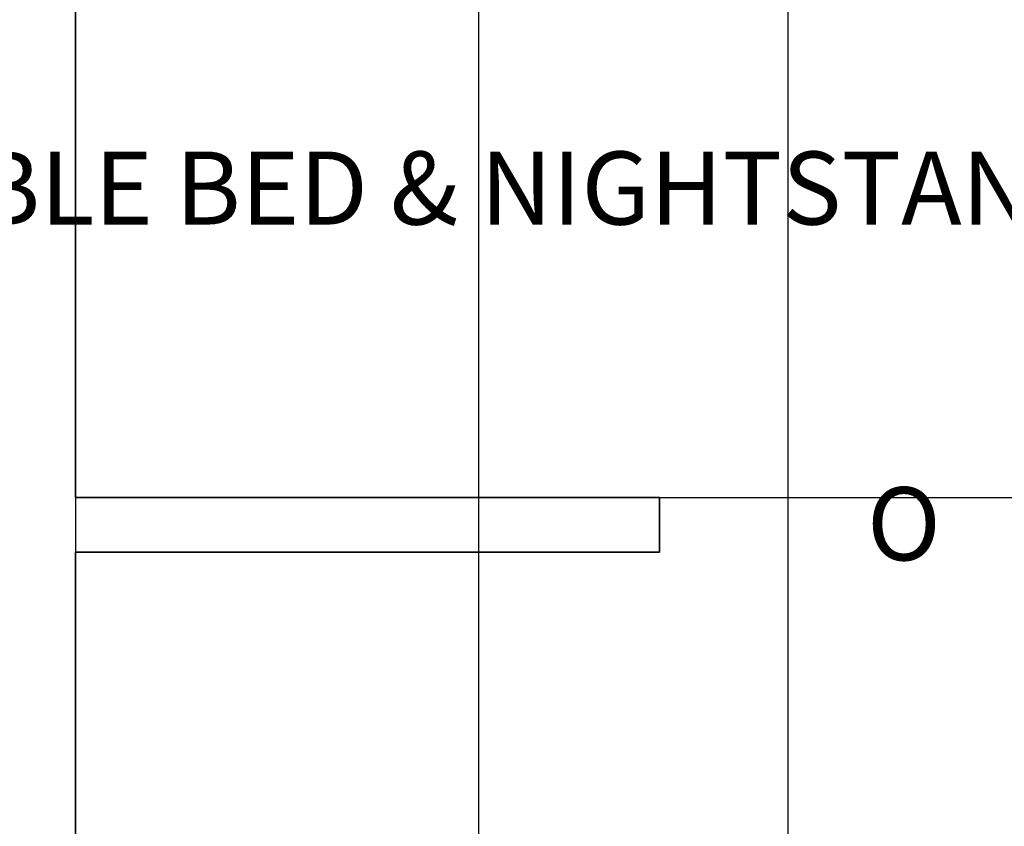
# Model space of a CAD drawing. Units: inches. Extents: x -26 to 575, y -18 to 513.
# Tile 21 of 28: x 274 to 355, y 307 to 374. Entities that reach past the tile are written whole.
import ezdxf

# ---------------------------------------------------------------- set-up
doc = ezdxf.new("R2010")
doc.units = ezdxf.units.IN
doc.header["$MEASUREMENT"] = 0
for name, color, linetype, lineweight in [('A-ANNO-DIMS', 2, 'Continuous', 18), ('A-ANNO-TEXT', 7, 'Continuous', 18), ('A-FLOR-CASE', 8, 'Continuous', 18), ('A-WALL', 7, 'Continuous', 35)]:
    doc.layers.add(name, color=color, linetype=linetype, lineweight=lineweight)
doc.styles.get("Standard").update_dxf_attribs({"font": 'arial.ttf', "height": 6})
doc.dimstyles.get("Standard").update_dxf_attribs({"dimtxt": 6, "dimasz": 0.18, "dimexe": 0.18, "dimexo": 0.0625, "dimgap": 0.09, "dimtad": 0, "dimtih": 1, "dimtoh": 1, "dimzin": 0, "dimdsep": 46, "dimlunit": 3, "dimtxsty": 'Standard', "dimcen": 0.09, "dimadec": 0, "dimazin": 0, "dimtfac": 1, "dimtofl": 0, "dimtmove": 0, "dimatfit": 3, "dimfxl": 1, "dimtolj": 1, "dimtzin": 0, "dimarcsym": 0})

# ---------------------------------------------------------------- blocks, each defined once
blk = doc.blocks.new('*D12')
at = {"layer": 'A-ANNO-DIMS', "color": 0, "lineweight": -2, "transparency": 16777216}
for p, q in [((143.378, 375.468), (143.378, 359.755)), ((247.348, 375.468), (247.348, 359.755)), ((143.558, 359.935), (247.168, 359.935)), ((247.348, 359.935), (247.528, 359.935))]:
    blk.add_line(p, q, dxfattribs=at)
at = {"layer": 'A-ANNO-DIMS', "color": 0, "transparency": 16777216}
for points in [[(143.558, 359.965), (143.558, 359.905), (143.378, 359.935)], [(247.168, 359.965), (247.168, 359.905), (247.348, 359.935)]]:
    blk.add_solid(points, dxfattribs=at)
at = {"layer": 'Defpoints', "color": 0, "transparency": 16777216}
for p in [(143.378, 375.531), (247.348, 375.531), (247.348, 359.935)]:
    blk.add_point(p, dxfattribs=at)
at = {"layer": 'A-ANNO-DIMS', "color": 0, "transparency": 16777216, "insert": (329.097, 359.935), "char_height": 6, "attachment_point": 5}
blk.add_mtext('\\A1;DOUBLE BED & NIGHTSTANDS 8\'-8" TYP.', dxfattribs=at)
blk = doc.blocks.new('*D31')
at = {"layer": 'A-ANNO-DIMS', "color": 0, "lineweight": -2, "transparency": 16777216}
for p, q in [((311.292, 466.445), (311.292, -8.972)), ((336.72, 466.445), (336.72, -8.972)), ((311.472, -8.792), (336.54, -8.792)), ((336.72, -8.792), (336.9, -8.792))]:
    blk.add_line(p, q, dxfattribs=at)
at = {"layer": 'A-ANNO-DIMS', "color": 0, "transparency": 16777216}
for points in [[(311.472, -8.762), (311.472, -8.822), (311.292, -8.792)], [(336.54, -8.762), (336.54, -8.822), (336.72, -8.792)]]:
    blk.add_solid(points, dxfattribs=at)
at = {"layer": 'Defpoints', "color": 0, "transparency": 16777216}
for p in [(311.292, 466.508), (336.72, 466.508), (336.72, -8.792)]:
    blk.add_point(p, dxfattribs=at)
at = {"layer": 'A-ANNO-DIMS', "color": 0, "transparency": 16777216, "insert": (352.006, -8.792), "char_height": 6, "attachment_point": 5}
blk.add_mtext('\\A1;2\'-1 1/2"', dxfattribs=at)
blk = doc.blocks.new('*D47')
at = {"layer": 'A-ANNO-DIMS', "color": 0, "lineweight": -2, "transparency": 16777216}
for p, q in [((278.177, 466.445), (278.177, -8.972)), ((311.292, 466.445), (311.292, -8.972)), ((278.357, -8.792), (286.619, -8.792)), ((311.112, -8.792), (302.851, -8.792))]:
    blk.add_line(p, q, dxfattribs=at)
at = {"layer": 'A-ANNO-DIMS', "color": 0, "transparency": 16777216}
for points in [[(278.357, -8.762), (278.357, -8.822), (278.177, -8.792)], [(311.112, -8.762), (311.112, -8.822), (311.292, -8.792)]]:
    blk.add_solid(points, dxfattribs=at)
at = {"layer": 'Defpoints', "color": 0, "transparency": 16777216}
for p in [(278.177, 466.508), (311.292, 466.508), (311.292, -8.792)]:
    blk.add_point(p, dxfattribs=at)
at = {"layer": 'A-ANNO-DIMS', "color": 0, "transparency": 16777216, "insert": (294.735, -8.792), "char_height": 6, "attachment_point": 5}
blk.add_mtext('\\A1;2\'-9"', dxfattribs=at)
blk = doc.blocks.new('*D49')
at = {"layer": 'A-ANNO-DIMS', "color": 0, "lineweight": -2, "transparency": 16777216}
for p, q in [((278.24, 466.508), (550.657, 466.508)), ((550.477, 466.328), (550.477, 403.661)), ((550.477, 334.688), (550.477, 397.355)), ((278.24, 334.508), (550.657, 334.508))]:
    blk.add_line(p, q, dxfattribs=at)
at = {"layer": 'A-ANNO-DIMS', "color": 0, "transparency": 16777216}
for points in [[(550.447, 466.328), (550.507, 466.328), (550.477, 466.508)], [(550.447, 334.688), (550.507, 334.688), (550.477, 334.508)]]:
    blk.add_solid(points, dxfattribs=at)
at = {"layer": 'Defpoints', "color": 0, "transparency": 16777216}
for p in [(278.177, 466.508), (550.477, 466.508), (278.177, 334.508)]:
    blk.add_point(p, dxfattribs=at)
at = {"layer": 'A-ANNO-DIMS', "color": 0, "transparency": 16777216, "insert": (550.477, 400.508), "char_height": 6, "attachment_point": 5}
blk.add_mtext('\\A1;11\'-0"', dxfattribs=at)

msp = doc.modelspace()

# ---------------------------------------------------------------- linework, layer by layer
at = {"layer": 'A-FLOR-CASE'}
msp.add_line((311.292, 334.508), (311.292, 466.508), dxfattribs=at)
at = {"layer": 'A-WALL'}
for p, q in [((278.177, 334.508), (278.177, 466.508)), ((326.177, 334.508), (278.177, 334.508)), ((326.177, 334.508), (326.177, 330.008)), ((278.177, 127.508), (278.177, 330.008)), ((326.177, 330.008), (278.177, 330.008))]:
    msp.add_line(p, q, dxfattribs=at)

# ---------------------------------------------------------------- texts
at = {"layer": 'A-ANNO-TEXT'}
msp.add_text('O', height=6, rotation=0.00167, dxfattribs=at).set_placement((343.237, 329.351))

# ---------------------------------------------------------------- dimensions: what is measured, and where the dimension line sits
at = {"layer": 'A-ANNO-DIMS'}
for base, p1, p2, picture, middle in [((311.292, -8.792), (278.177, 466.508), (311.292, 466.508), '*D47', (294.735, -8.792)), ((336.72, -8.792), (311.292, 466.508), (336.72, 466.508), '*D31', (352.006, -8.792))]:
    dim = msp.add_linear_dim(base=base, p1=p1, p2=p2, dimstyle='Standard', override={"dimdec": 1, "dimlfac": 1, "dimrnd": 0, "dimzin": 1, "dimdsep": 46, "dimlunit": 4, "dimfrac": 2}, dxfattribs=at)
    dim.commit()
    dim.dimension.update_dxf_attribs({"geometry": picture, "text_midpoint": middle})
dim = msp.add_linear_dim(base=(550.477, 466.508), p1=(278.177, 334.508), p2=(278.177, 466.508), angle=90, dimstyle='Standard', override={"dimdec": 1, "dimlfac": 1, "dimrnd": 0, "dimzin": 1, "dimdsep": 46, "dimlunit": 4, "dimfrac": 2}, dxfattribs=at)
dim.commit()
dim.dimension.update_dxf_attribs({"geometry": '*D49', "text_midpoint": (550.477, 400.508)})
dim = msp.add_linear_dim(base=(247.348, 359.935), p1=(143.378, 375.531), p2=(247.348, 375.531), text='DOUBLE BED & NIGHTSTANDS <> TYP.', dimstyle='Standard', override={"dimdec": 1, "dimlfac": 1, "dimrnd": 0, "dimzin": 1, "dimdsep": 46, "dimlunit": 4, "dimfrac": 2}, dxfattribs=at)
dim.commit()
dim.dimension.update_dxf_attribs({"geometry": '*D12', "text_midpoint": (329.097, 359.935)})

doc.saveas('drawing.dxf')
